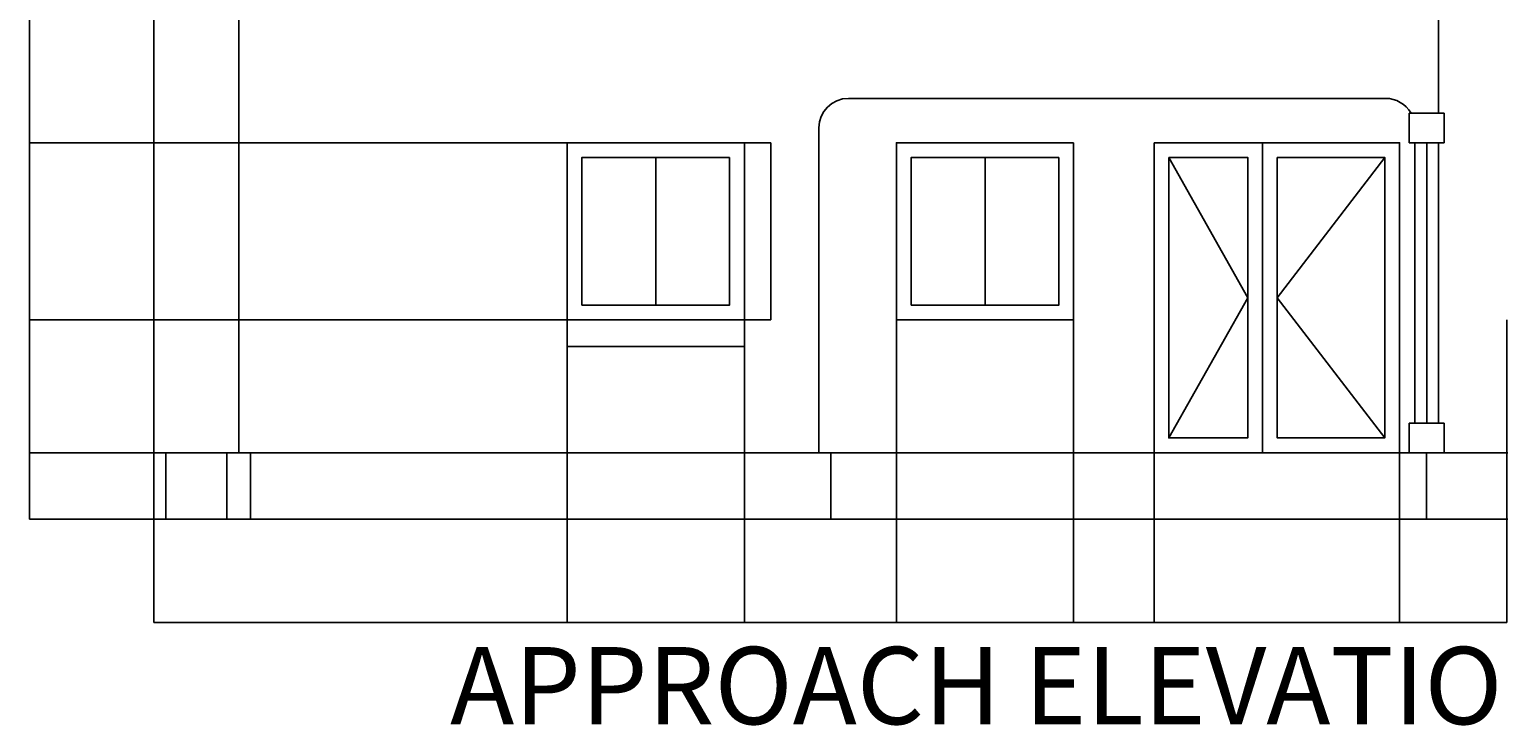
# Model space of a CAD drawing. Units: millimetres. Extents: x 19292 to 100733, y 12374 to 26974.
# Tile 24 of 24: x 85594 to 95547, y 13711 to 18427. Entities that reach past the tile are written whole.
import ezdxf

# ---------------------------------------------------------------- set-up
doc = ezdxf.new("R2010")
doc.units = ezdxf.units.MM
for name, color, linetype, lineweight in [('A-ANNO-DIMS', 2, 'Continuous', 18), ('A-ANNO-TEXT', 7, 'Continuous', 35), ('A-ELEV', 7, 'Continuous', 25)]:
    doc.layers.add(name, color=color, linetype=linetype, lineweight=lineweight)
doc.styles.get("Standard").update_dxf_attribs({"font": 'arial.ttf'})
doc.dimstyles.get("Standard").update_dxf_attribs({"dimtxt": 0.18, "dimasz": 0.18, "dimexe": 0.18, "dimexo": 0.0625, "dimgap": 0.09, "dimtad": 0, "dimtih": 1, "dimtoh": 1, "dimdec": 4, "dimzin": 0, "dimdsep": 46, "dimtxsty": 'Standard', "dimcen": 0.09, "dimadec": 0, "dimazin": 0, "dimtfac": 1, "dimtdec": 4, "dimtofl": 0, "dimtmove": 0, "dimatfit": 3, "dimfxl": 1, "dimtolj": 1, "dimtzin": 0, "dimarcsym": 0})

# ---------------------------------------------------------------- blocks, each defined once
blk = doc.blocks.new('WIN-ELEV-1200')
blk.add_line((599.9999832836038, 1100.000156100592), (599.9999832836038, 100.000156100592))
for points in [[(1199.999983283604, 1200.000156100592), (1199.999983283604, 0.0001561005919939), (-1.67163962033e-05, 0.0001561005919939), (-1.67163962033e-05, 1200.000156100592)], [(1099.999983283604, 1100.000156100592), (1099.999983283604, 100.000156100592), (99.9999832836038, 100.000156100592), (99.9999832836038, 1100.000156100592)]]:
    blk.add_lwpolyline(points, close=True)
blk = doc.blocks.new('*D56')
at = {"layer": 'A-ANNO-DIMS', "color": 0, "lineweight": -2, "transparency": 16777216}
for p, q in [((89237.01698328361, 16459.84665610059), (89237.01698328361, 16279.72915610059)), ((90437.0169832836, 16459.84665610059), (90437.0169832836, 16279.72915610059)), ((89237.1969832836, 16279.90915610059), (89835.44413198755, 16279.90915610059)), ((90436.8369832836, 16279.90915610059), (89838.58983457964, 16279.90915610059))]:
    blk.add_line(p, q, dxfattribs=at)
at = {"layer": 'A-ANNO-DIMS', "color": 0, "transparency": 16777216}
for points in [[(89237.1969832836, 16279.93915610059), (89237.1969832836, 16279.87915610059), (89237.01698328361, 16279.90915610059)], [(90436.8369832836, 16279.93915610059), (90436.8369832836, 16279.87915610059), (90437.0169832836, 16279.90915610059)]]:
    blk.add_solid(points, dxfattribs=at)
at = {"layer": 'Defpoints', "color": 0, "transparency": 16777216}
for p in [(89237.01698328361, 16459.90915610059), (90437.0169832836, 16459.90915610059), (90437.0169832836, 16279.90915610059)]:
    blk.add_point(p, dxfattribs=at)
at = {"layer": 'A-ANNO-DIMS', "color": 0, "transparency": 16777216, "insert": (89837.0169832836, 16279.90915610059), "char_height": 0.18, "attachment_point": 5}
blk.add_mtext('\\A1;WINDOW 1200 1200 TYP.', dxfattribs=at)
blk = doc.blocks.new('*D57')
at = {"layer": 'A-ANNO-DIMS', "color": 0, "lineweight": -2, "transparency": 16777216}
for p, q in [((90437.07948328363, 17659.9091561006), (90617.19698328365, 17659.9091561006)), ((90617.01698328365, 17659.7291561006), (90617.01698328365, 17060.09105923839)), ((90617.01698328365, 16460.0891561006), (90617.01698328365, 17059.72725296281)), ((90437.07948328363, 16459.9091561006), (90617.19698328365, 16459.9091561006))]:
    blk.add_line(p, q, dxfattribs=at)
at = {"layer": 'A-ANNO-DIMS', "color": 0, "transparency": 16777216}
for points in [[(90616.98698328366, 17659.7291561006), (90617.04698328365, 17659.7291561006), (90617.01698328365, 17659.9091561006)], [(90616.98698328366, 16460.0891561006), (90617.04698328365, 16460.0891561006), (90617.01698328365, 16459.9091561006)]]:
    blk.add_solid(points, dxfattribs=at)
at = {"layer": 'Defpoints', "color": 0, "transparency": 16777216}
for p in [(90437.01698328363, 17659.9091561006), (90617.01698328365, 17659.9091561006), (90437.01698328363, 16459.9091561006)]:
    blk.add_point(p, dxfattribs=at)
at = {"layer": 'A-ANNO-DIMS', "color": 0, "transparency": 16777216, "insert": (90617.01698328365, 17059.90915610057), "char_height": 0.18, "attachment_point": 5}
blk.add_mtext('\\A1;1200 TYP.', dxfattribs=at)
blk = doc.blocks.new('*D141')
at = {"layer": 'A-ANNO-DIMS', "color": 0, "lineweight": -2, "transparency": 16777216}
for p, q in [((86437.75175800003, 15559.909156), (85593.98509100005, 15559.909156)), ((85594.16509100008, 15559.729156), (85594.16509100008, 15335.09105913779)), ((85594.16509100008, 15110.089156), (85594.16509100008, 15334.72725286221)), ((86437.75175800003, 15109.909156), (85593.98509100005, 15109.909156))]:
    blk.add_line(p, q, dxfattribs=at)
at = {"layer": 'A-ANNO-DIMS', "color": 0, "transparency": 16777216}
for points in [[(85594.13509100005, 15559.729156), (85594.19509100006, 15559.729156), (85594.16509100008, 15559.909156)], [(85594.13509100005, 15110.089156), (85594.19509100006, 15110.089156), (85594.16509100008, 15109.909156)]]:
    blk.add_solid(points, dxfattribs=at)
at = {"layer": 'Defpoints', "color": 0, "transparency": 16777216}
for p in [(85594.16509100008, 15559.909156), (86437.81425800003, 15559.909156), (86437.81425800003, 15109.909156)]:
    blk.add_point(p, dxfattribs=at)
at = {"layer": 'A-ANNO-DIMS', "color": 0, "transparency": 16777216, "insert": (85594.16509100005, 15334.90915599998), "char_height": 0.18, "attachment_point": 5}
blk.add_mtext('\\A1;450', dxfattribs=at)
blk = doc.blocks.new('*D142')
at = {"layer": 'A-ANNO-DIMS', "color": 0, "lineweight": -2, "transparency": 16777216}
for p, q in [((89236.95448300001, 16459.90915600001), (85593.98509100005, 16459.90915600001)), ((85594.16509100008, 16459.72915600001), (85594.16509100008, 16010.09105913779)), ((85594.16509100008, 15560.089156), (85594.16509100008, 16009.72725286221)), ((86437.75175800003, 15559.909156), (85593.98509100005, 15559.909156))]:
    blk.add_line(p, q, dxfattribs=at)
at = {"layer": 'A-ANNO-DIMS', "color": 0, "transparency": 16777216}
for points in [[(85594.13509100005, 16459.72915600001), (85594.19509100006, 16459.72915600001), (85594.16509100008, 16459.90915600001)], [(85594.13509100005, 15560.089156), (85594.19509100006, 15560.089156), (85594.16509100008, 15559.909156)]]:
    blk.add_solid(points, dxfattribs=at)
at = {"layer": 'Defpoints', "color": 0, "transparency": 16777216}
for p in [(85594.16509100008, 16459.90915600001), (89237.01698300002, 16459.90915600001), (86437.81425800003, 15559.909156)]:
    blk.add_point(p, dxfattribs=at)
at = {"layer": 'A-ANNO-DIMS', "color": 0, "transparency": 16777216, "insert": (85594.16509100005, 16009.90915599998), "char_height": 0.18, "attachment_point": 5}
blk.add_mtext('\\A1;900', dxfattribs=at)
blk = doc.blocks.new('*D143')
at = {"layer": 'A-ANNO-DIMS', "color": 0, "lineweight": -2, "transparency": 16777216}
for p, q in [((89236.95448300001, 17659.90915600001), (85593.98509100005, 17659.90915600001)), ((85594.16509100008, 17659.72915600001), (85594.16509100008, 17060.0910591378)), ((85594.16509100008, 16460.08915600001), (85594.16509100008, 17059.72725286222)), ((89236.95448300001, 16459.90915600001), (85593.98509100005, 16459.90915600001))]:
    blk.add_line(p, q, dxfattribs=at)
at = {"layer": 'A-ANNO-DIMS', "color": 0, "transparency": 16777216}
for points in [[(85594.13509100005, 17659.72915600001), (85594.19509100006, 17659.72915600001), (85594.16509100008, 17659.90915600001)], [(85594.13509100005, 16460.08915600001), (85594.19509100006, 16460.08915600001), (85594.16509100008, 16459.90915600001)]]:
    blk.add_solid(points, dxfattribs=at)
at = {"layer": 'Defpoints', "color": 0, "transparency": 16777216}
for p in [(85594.16509100008, 17659.90915600001), (89237.01698300002, 17659.90915600001), (89237.01698300002, 16459.90915600001)]:
    blk.add_point(p, dxfattribs=at)
at = {"layer": 'A-ANNO-DIMS', "color": 0, "transparency": 16777216, "insert": (85594.16509100005, 17059.90915599998), "char_height": 0.18, "attachment_point": 5}
blk.add_mtext('\\A1;1200', dxfattribs=at)
blk = doc.blocks.new('*D144')
at = {"layer": 'A-ANNO-DIMS', "color": 0, "lineweight": -2, "transparency": 16777216}
for p, q in [((89121.76770300003, 19459.90915600001), (85593.98509100005, 19459.90915600001)), ((85594.16509100008, 19459.72915600001), (85594.16509100008, 18560.0910591378)), ((85594.16509100008, 17660.08915600001), (85594.16509100008, 18559.72725286222)), ((89236.95448300001, 17659.90915600001), (85593.98509100005, 17659.90915600001))]:
    blk.add_line(p, q, dxfattribs=at)
at = {"layer": 'A-ANNO-DIMS', "color": 0, "transparency": 16777216}
for points in [[(85594.13509100005, 19459.72915600001), (85594.19509100006, 19459.72915600001), (85594.16509100008, 19459.90915600001)], [(85594.13509100005, 17660.08915600001), (85594.19509100006, 17660.08915600001), (85594.16509100008, 17659.90915600001)]]:
    blk.add_solid(points, dxfattribs=at)
at = {"layer": 'Defpoints', "color": 0, "transparency": 16777216}
for p in [(85594.16509100008, 19459.90915600001), (89121.83020300003, 19459.90915600001), (89237.01698300002, 17659.90915600001)]:
    blk.add_point(p, dxfattribs=at)
at = {"layer": 'A-ANNO-DIMS', "color": 0, "transparency": 16777216, "insert": (85594.16509100005, 18559.90915599998), "char_height": 0.18, "attachment_point": 5}
blk.add_mtext('\\A1;1800', dxfattribs=at)
blk = doc.blocks.new('*D151')
at = {"layer": 'A-ANNO-DIMS', "color": 0, "lineweight": -2, "transparency": 16777216}
for p, q in [((91039.56247500001, 26274.21100900001), (100732.6942110001, 26274.21100900001)), ((100732.5142110001, 26274.03100900001), (100732.5142110001, 20692.2419856378)), ((100732.5142110001, 15110.08915600001), (100732.5142110001, 20691.87817936222)), ((99927.91327500006, 15109.909156), (100732.6942110001, 15109.909156))]:
    blk.add_line(p, q, dxfattribs=at)
at = {"layer": 'A-ANNO-DIMS', "color": 0, "transparency": 16777216}
for points in [[(100732.4842110001, 26274.03100900001), (100732.5442110001, 26274.03100900001), (100732.5142110001, 26274.21100900001)], [(100732.4842110001, 15110.08915600001), (100732.5442110001, 15110.08915600001), (100732.5142110001, 15109.909156)]]:
    blk.add_solid(points, dxfattribs=at)
at = {"layer": 'Defpoints', "color": 0, "transparency": 16777216}
for p in [(91039.49997500001, 26274.21100900001), (100732.5142110001, 26274.21100900001), (99927.85077500006, 15109.909156)]:
    blk.add_point(p, dxfattribs=at)
at = {"layer": 'A-ANNO-DIMS', "color": 0, "transparency": 16777216, "insert": (100732.5142110001, 20692.06008249997), "char_height": 0.18, "attachment_point": 5}
blk.add_mtext('\\A1;11164', dxfattribs=at)
blk = doc.blocks.new('*D152')
at = {"layer": 'A-ANNO-DIMS', "color": 0, "lineweight": -2, "transparency": 16777216}
for p, q in [((89237.016983, 16459.846656), (89237.016983, 14409.716173)), ((86437.814258, 15559.846656), (86437.814258, 14409.716173)), ((86437.99425799999, 14409.896173), (87837.05512936765, 14409.896173)), ((89236.83698300002, 14409.896173), (87837.77611163232, 14409.896173))]:
    blk.add_line(p, q, dxfattribs=at)
at = {"layer": 'A-ANNO-DIMS', "color": 0, "transparency": 16777216}
for points in [[(86437.99425799999, 14409.926173), (86437.99425799999, 14409.866173), (86437.814258, 14409.896173)], [(89236.83698300002, 14409.926173), (89236.83698300002, 14409.866173), (89237.016983, 14409.896173)]]:
    blk.add_solid(points, dxfattribs=at)
at = {"layer": 'Defpoints', "color": 0, "transparency": 16777216}
for p in [(89237.016983, 16459.909156), (86437.814258, 15559.909156), (89237.016983, 14409.896173)]:
    blk.add_point(p, dxfattribs=at)
at = {"layer": 'A-ANNO-DIMS', "color": 0, "transparency": 16777216, "insert": (87837.41562049997, 14409.896173), "char_height": 0.18, "attachment_point": 5}
blk.add_mtext('\\A1;2799', dxfattribs=at)
blk = doc.blocks.new('*D153')
at = {"layer": 'A-ANNO-DIMS', "color": 0, "lineweight": -2, "transparency": 16777216}
for p, q in [((89237.016983, 16459.846656), (89237.016983, 14409.716173)), ((90437.016983, 16459.846656), (90437.016983, 14409.716173)), ((89237.19698299999, 14409.896173), (89836.66698982126, 14409.896173)), ((90436.836983, 14409.896173), (89837.36697617872, 14409.896173))]:
    blk.add_line(p, q, dxfattribs=at)
at = {"layer": 'A-ANNO-DIMS', "color": 0, "transparency": 16777216}
for points in [[(89237.19698299999, 14409.926173), (89237.19698299999, 14409.866173), (89237.016983, 14409.896173)], [(90436.836983, 14409.926173), (90436.836983, 14409.866173), (90437.016983, 14409.896173)]]:
    blk.add_solid(points, dxfattribs=at)
at = {"layer": 'Defpoints', "color": 0, "transparency": 16777216}
for p in [(89237.016983, 16459.909156), (90437.016983, 16459.909156), (90437.016983, 14409.896173)]:
    blk.add_point(p, dxfattribs=at)
at = {"layer": 'A-ANNO-DIMS', "color": 0, "transparency": 16777216, "insert": (89837.016983, 14409.896173), "char_height": 0.18, "attachment_point": 5}
blk.add_mtext('\\A1;1200', dxfattribs=at)
blk = doc.blocks.new('*D154')
at = {"layer": 'A-ANNO-DIMS', "color": 0, "lineweight": -2, "transparency": 16777216}
for p, q in [((90437.016983, 16459.846656), (90437.016983, 14409.716173)), ((91467.756632, 16459.846656), (91467.756632, 14409.716173)), ((90437.19698299999, 14409.896173), (90951.93165061051, 14409.896173)), ((91467.576632, 14409.896173), (90952.84196438949, 14409.896173))]:
    blk.add_line(p, q, dxfattribs=at)
at = {"layer": 'A-ANNO-DIMS', "color": 0, "transparency": 16777216}
for points in [[(90437.19698299999, 14409.926173), (90437.19698299999, 14409.866173), (90437.016983, 14409.896173)], [(91467.576632, 14409.926173), (91467.576632, 14409.866173), (91467.756632, 14409.896173)]]:
    blk.add_solid(points, dxfattribs=at)
at = {"layer": 'Defpoints', "color": 0, "transparency": 16777216}
for p in [(90437.016983, 16459.909156), (91467.756632, 16459.909156), (91467.756632, 14409.896173)]:
    blk.add_point(p, dxfattribs=at)
at = {"layer": 'A-ANNO-DIMS', "color": 0, "transparency": 16777216, "insert": (90952.3868075, 14409.896173), "char_height": 0.18, "attachment_point": 5}
blk.add_mtext('\\A1;1030.7', dxfattribs=at)
blk = doc.blocks.new('*D155')
at = {"layer": 'A-ANNO-DIMS', "color": 0, "lineweight": -2, "transparency": 16777216}
for p, q in [((91467.756632, 16459.846656), (91467.756632, 14409.716173)), ((92667.756632, 16459.846656), (92667.756632, 14409.716173)), ((91467.936632, 14409.896173), (92067.40663882127, 14409.896173)), ((92667.57663200001, 14409.896173), (92068.10662517873, 14409.896173))]:
    blk.add_line(p, q, dxfattribs=at)
at = {"layer": 'A-ANNO-DIMS', "color": 0, "transparency": 16777216}
for points in [[(91467.936632, 14409.926173), (91467.936632, 14409.866173), (91467.756632, 14409.896173)], [(92667.57663200001, 14409.926173), (92667.57663200001, 14409.866173), (92667.756632, 14409.896173)]]:
    blk.add_solid(points, dxfattribs=at)
at = {"layer": 'Defpoints', "color": 0, "transparency": 16777216}
for p in [(91467.756632, 16459.909156), (92667.756632, 16459.909156), (92667.756632, 14409.896173)]:
    blk.add_point(p, dxfattribs=at)
at = {"layer": 'A-ANNO-DIMS', "color": 0, "transparency": 16777216, "insert": (92067.756632, 14409.896173), "char_height": 0.18, "attachment_point": 5}
blk.add_mtext('\\A1;1200', dxfattribs=at)
blk = doc.blocks.new('*D156')
at = {"layer": 'A-ANNO-DIMS', "color": 0, "lineweight": -2, "transparency": 16777216}
for p, q in [((92667.756632, 16459.846656), (92667.756632, 14409.716173)), ((93212.252828, 15559.846656), (93212.252828, 14409.716173)), ((92667.936632, 14409.896173), (92939.6103507367, 14409.896173)), ((93212.072828, 14409.896173), (92940.39910926331, 14409.896173))]:
    blk.add_line(p, q, dxfattribs=at)
at = {"layer": 'A-ANNO-DIMS', "color": 0, "transparency": 16777216}
for points in [[(92667.936632, 14409.926173), (92667.936632, 14409.866173), (92667.756632, 14409.896173)], [(93212.072828, 14409.926173), (93212.072828, 14409.866173), (93212.252828, 14409.896173)]]:
    blk.add_solid(points, dxfattribs=at)
at = {"layer": 'Defpoints', "color": 0, "transparency": 16777216}
for p in [(92667.756632, 16459.909156), (93212.252828, 15559.909156), (93212.252828, 14409.896173)]:
    blk.add_point(p, dxfattribs=at)
at = {"layer": 'A-ANNO-DIMS', "color": 0, "transparency": 16777216, "insert": (92940.00473, 14409.896173), "char_height": 0.18, "attachment_point": 5}
blk.add_mtext('\\A1;544.5', dxfattribs=at)
blk = doc.blocks.new('*D157')
at = {"layer": 'A-ANNO-DIMS', "color": 0, "lineweight": -2, "transparency": 16777216}
for p, q in [((93212.252828, 15559.846656), (93212.252828, 14409.716173)), ((94875.223652, 15559.846656), (94875.223652, 14409.716173)), ((93212.43282799999, 14409.896173), (94043.38793986358, 14409.896173)), ((94875.04365200001, 14409.896173), (94044.08854013644, 14409.896173))]:
    blk.add_line(p, q, dxfattribs=at)
at = {"layer": 'A-ANNO-DIMS', "color": 0, "transparency": 16777216}
for points in [[(93212.43282799999, 14409.926173), (93212.43282799999, 14409.866173), (93212.252828, 14409.896173)], [(94875.04365200001, 14409.926173), (94875.04365200001, 14409.866173), (94875.223652, 14409.896173)]]:
    blk.add_solid(points, dxfattribs=at)
at = {"layer": 'Defpoints', "color": 0, "transparency": 16777216}
for p in [(93212.252828, 15559.909156), (94875.223652, 15559.909156), (94875.223652, 14409.896173)]:
    blk.add_point(p, dxfattribs=at)
at = {"layer": 'A-ANNO-DIMS', "color": 0, "transparency": 16777216, "insert": (94043.73824, 14409.896173), "char_height": 0.18, "attachment_point": 5}
blk.add_mtext('\\A1;1663', dxfattribs=at)
blk = doc.blocks.new('*D158')
at = {"layer": 'A-ANNO-DIMS', "color": 0, "lineweight": -2, "transparency": 16777216}
for p, q in [((95602.426915, 16459.846656), (95602.426915, 14409.716173)), ((94875.223652, 15559.846656), (94875.223652, 14409.716173)), ((94875.403652, 14409.896173), (95238.43323711529, 14409.896173)), ((95602.24691500001, 14409.896173), (95239.21732988473, 14409.896173))]:
    blk.add_line(p, q, dxfattribs=at)
at = {"layer": 'A-ANNO-DIMS', "color": 0, "transparency": 16777216}
for points in [[(94875.403652, 14409.926173), (94875.403652, 14409.866173), (94875.223652, 14409.896173)], [(95602.24691500001, 14409.926173), (95602.24691500001, 14409.866173), (95602.426915, 14409.896173)]]:
    blk.add_solid(points, dxfattribs=at)
at = {"layer": 'Defpoints', "color": 0, "transparency": 16777216}
for p in [(95602.426915, 16459.909156), (94875.223652, 15559.909156), (95602.426915, 14409.896173)]:
    blk.add_point(p, dxfattribs=at)
at = {"layer": 'A-ANNO-DIMS', "color": 0, "transparency": 16777216, "insert": (95238.8252835, 14409.896173), "char_height": 0.18, "attachment_point": 5}
blk.add_mtext('\\A1;727.2', dxfattribs=at)

msp = doc.modelspace()

# ---------------------------------------------------------------- linework, layer by layer
at = {"layer": 'A-ELEV'}
for p, q in [((87012.49645682552, 15559.90915610059), (87012.49645682552, 21559.90915610059)), ((86437.81425804387, 15559.90915610059), (86437.81425804387, 18559.90915610059)), ((95138.48032185201, 17859.90915610059), (95138.48032185201, 18559.90915610059)), ((91142.49645682552, 17959.90915610059), (94780.02868698302, 17959.90915610059)), ((94940.02868698297, 17659.90915610059), (94940.02868698297, 17859.90915610059)), ((94940.02868698297, 17859.90915610059), (95178.480321852, 17859.90915610059)), ((95178.48032185201, 17659.90915610059), (95178.48032185201, 17859.90915610059)), ((90942.49645682554, 15559.90915610059), (90942.49645682554, 17759.90915610059)), ((94940.02868698297, 17659.90915610059), (95178.480321852, 17659.90915610059)), ((94980.02868698302, 15759.90915610059), (94980.02868698302, 17659.90915610059)), ((95059.25450441749, 17659.90915610059), (95059.2545044175, 15759.90915610059)), ((95138.48032185201, 15759.90915610059), (95138.48032185201, 17659.90915610059)), ((93312.252827786, 17559.90915610059), (93847.52488627864, 16609.90915610059)), ((94775.22365204261, 17559.90915610059), (94047.52488627862, 16609.90915610059)), ((93847.52488627864, 16609.90915610059), (93312.252827786, 15659.90915610059)), ((94047.52488627862, 16609.90915610059), (94775.22365204261, 15659.90915610059)), ((94940.02868698302, 15559.90915610059), (94940.02868698302, 15759.90915610059)), ((94940.028686983, 15759.90915610059), (95178.48032185201, 15759.90915610059)), ((95178.48032185201, 15559.90915610059), (95178.48032185201, 15759.90915610059)), ((86437.81425804387, 15559.90915610059), (99927.85077479901, 15559.90915610059)), ((86517.81425804387, 15109.90915610059), (86517.81425804387, 15559.90915610059)), ((86932.49645682554, 15109.90915610059), (86932.49645682554, 15559.90915610059)), ((87092.49645682554, 15109.90915610059), (87092.49645682554, 15559.90915610059)), ((91022.49645682555, 15109.90915610059), (91022.49645682555, 15559.90915610059)), ((95058.480321852, 15109.90915610059), (95058.480321852, 15559.90915610059)), ((86437.81425804387, 15109.90915610059), (99927.85077479901, 15109.90915610059))]:
    msp.add_line(p, q, dxfattribs=at)
for points in [[(93212.252827786, 17659.90915610059), (93947.52488627862, 17659.90915610059), (93947.52488627862, 15559.90915610059), (93212.252827786, 15559.90915610059)], [(93947.52488627862, 17659.90915610059), (94875.22365204261, 17659.90915610059), (94875.22365204261, 15559.90915610059), (93947.52488627862, 15559.90915610059)], [(93312.252827786, 17559.90915610059), (93847.52488627864, 17559.90915610059), (93847.52488627864, 15659.90915610059), (93312.252827786, 15659.90915610059)], [(94047.52488627862, 17559.90915610059), (94775.22365204261, 17559.90915610059), (94775.22365204261, 15659.90915610059), (94047.52488627862, 15659.90915610059)]]:
    msp.add_lwpolyline(points, close=True, dxfattribs=at)
for centre, start, end in [((91142.49645682552, 17759.90915610059), 90, 180), ((94780.02868698302, 17759.90915610059), 30.00000000009106, 90)]:
    msp.add_arc(centre, 200, start, end, dxfattribs=at)

# ---------------------------------------------------------------- block references
for p in [(89237.017, 16459.909), (91467.75664892825, 16459.909)]:
    msp.add_blockref('WIN-ELEV-1200', p, dxfattribs=at)

# ---------------------------------------------------------------- texts
at = {"layer": 'A-ANNO-TEXT'}
msp.add_text('APPROACH ELEVATION', height=523.2684807306957, dxfattribs=at).set_placement((88444.08516921198, 13720.60677981616))

# ---------------------------------------------------------------- dimensions: what is measured, and where the dimension line sits
at = {"layer": 'A-ANNO-DIMS'}
for base, p1, p2, picture, middle in [((100732.5142110001, 26274.21100900001), (99927.850775, 15109.909156), (91039.499975, 26274.211009), '*D151', (100732.5142110001, 20692.06008249997)), ((85594.16509100008, 19459.90915600001), (89237.016983, 17659.909156), (89121.830203, 19459.909156), '*D144', (85594.16509100005, 18559.90915599998)), ((85594.16509100008, 17659.90915600001), (89237.016983, 16459.909156), (89237.016983, 17659.909156), '*D143', (85594.16509100005, 17059.90915599998)), ((85594.16509100008, 16459.90915600001), (86437.814258, 15559.909156), (89237.016983, 16459.909156), '*D142', (85594.16509100005, 16009.90915599998)), ((85594.16509100008, 15559.909156), (86437.814258, 15109.909156), (86437.814258, 15559.909156), '*D141', (85594.16509100005, 15334.90915599998))]:
    dim = msp.add_linear_dim(base=base, p1=p1, p2=p2, angle=90, dimstyle='Standard', override={"dimdec": 0, "dimlfac": 1, "dimrnd": 0, "dimzin": 0, "dimdsep": 46, "dimlunit": 2}, dxfattribs=at)
    dim.commit()
    dim.dimension.update_dxf_attribs({"geometry": picture, "text_midpoint": middle})
dim = msp.add_linear_dim(base=(90617.01698328365, 17659.9091561006), p1=(90437.0169832836, 16459.90915610059), p2=(90437.0169832836, 17659.90915610059), angle=90, text='<> TYP.', dimstyle='Standard', override={"dimdec": 0, "dimrnd": 0, "dimzin": 0, "dimlunit": 2}, dxfattribs=at)
dim.commit()
dim.dimension.update_dxf_attribs({"geometry": '*D57', "text_midpoint": (90617.01698328365, 17059.90915610057)})
for base, p1, p2, override, picture, middle in [((89237.016983, 14409.896173), (86437.814258, 15559.909156), (89237.016983, 16459.909156), {"dimdec": 0, "dimlfac": 1, "dimrnd": 0, "dimzin": 0, "dimdsep": 46, "dimlunit": 2}, '*D152', (87837.41562049997, 14409.896173)), ((90437.016983, 14409.896173), (89237.016983, 16459.909156), (90437.016983, 16459.909156), {"dimdec": 0, "dimlfac": 1, "dimrnd": 0, "dimzin": 0, "dimdsep": 46, "dimlunit": 2}, '*D153', (89837.016983, 14409.896173)), ((91467.756632, 14409.896173), (90437.016983, 16459.909156), (91467.756632, 16459.909156), {"dimdec": 1, "dimlfac": 1, "dimrnd": 0, "dimzin": 0, "dimdsep": 46, "dimlunit": 2}, '*D154', (90952.3868075, 14409.896173)), ((92667.756632, 14409.896173), (91467.756632, 16459.909156), (92667.756632, 16459.909156), {"dimdec": 0, "dimlfac": 1, "dimrnd": 0, "dimzin": 0, "dimdsep": 46, "dimlunit": 2}, '*D155', (92067.756632, 14409.896173)), ((93212.252828, 14409.896173), (92667.756632, 16459.909156), (93212.252828, 15559.909156), {"dimdec": 1, "dimlfac": 1, "dimrnd": 0, "dimzin": 0, "dimdsep": 46, "dimlunit": 2}, '*D156', (92940.00473, 14409.896173)), ((95602.426915, 14409.896173), (94875.223652, 15559.909156), (95602.426915, 16459.909156), {"dimdec": 1, "dimlfac": 1, "dimrnd": 0, "dimzin": 0, "dimdsep": 46, "dimlunit": 2}, '*D158', (95238.8252835, 14409.896173)), ((94875.223652, 14409.896173), (93212.252828, 15559.909156), (94875.223652, 15559.909156), {"dimdec": 0, "dimlfac": 1, "dimrnd": 0, "dimzin": 0, "dimdsep": 46, "dimlunit": 2}, '*D157', (94043.73824, 14409.896173))]:
    dim = msp.add_linear_dim(base=base, p1=p1, p2=p2, dimstyle='Standard', override=override, dxfattribs=at)
    dim.commit()
    dim.dimension.update_dxf_attribs({"geometry": picture, "text_midpoint": middle})
dim = msp.add_linear_dim(base=(90437.0169832836, 16279.90915610059), p1=(89237.01698328361, 16459.90915610059), p2=(90437.0169832836, 16459.90915610059), text='WINDOW 1200 <> TYP.', dimstyle='Standard', override={"dimdec": 0, "dimrnd": 0, "dimzin": 0, "dimlunit": 2}, dxfattribs=at)
dim.commit()
dim.dimension.update_dxf_attribs({"geometry": '*D56', "text_midpoint": (89837.0169832836, 16279.90915610059)})

doc.saveas('drawing.dxf')
